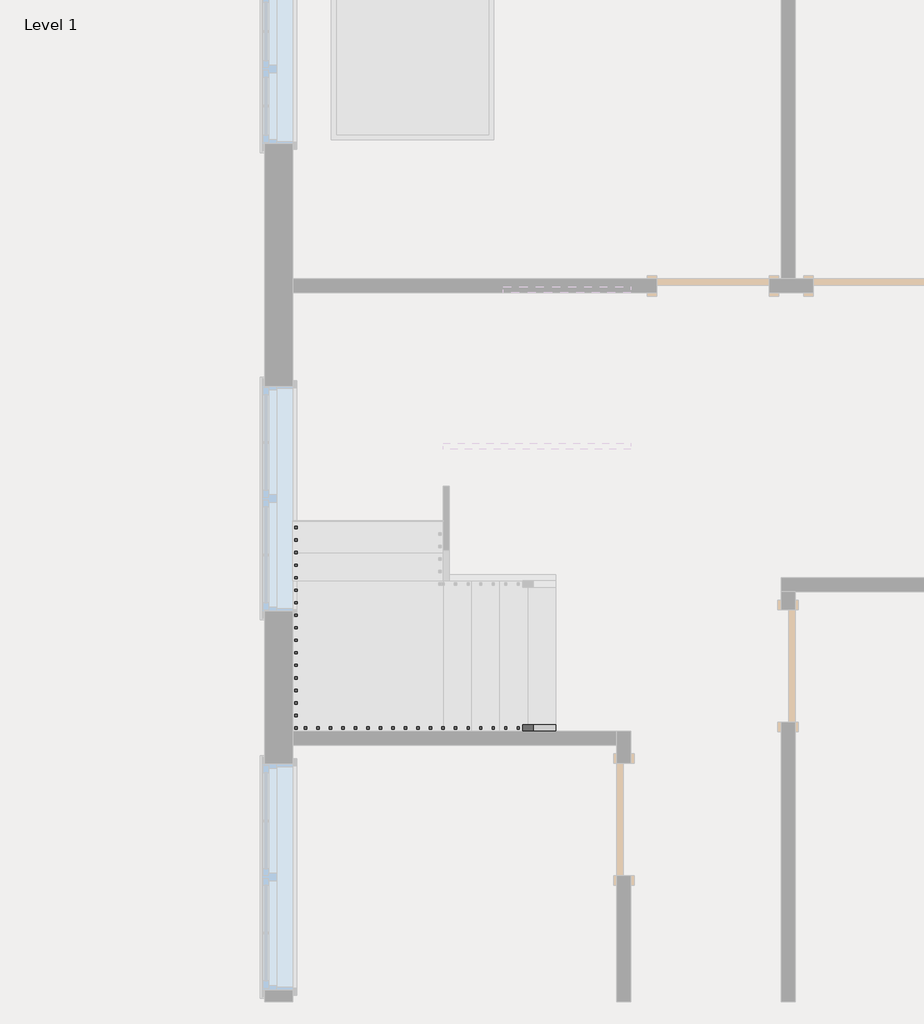
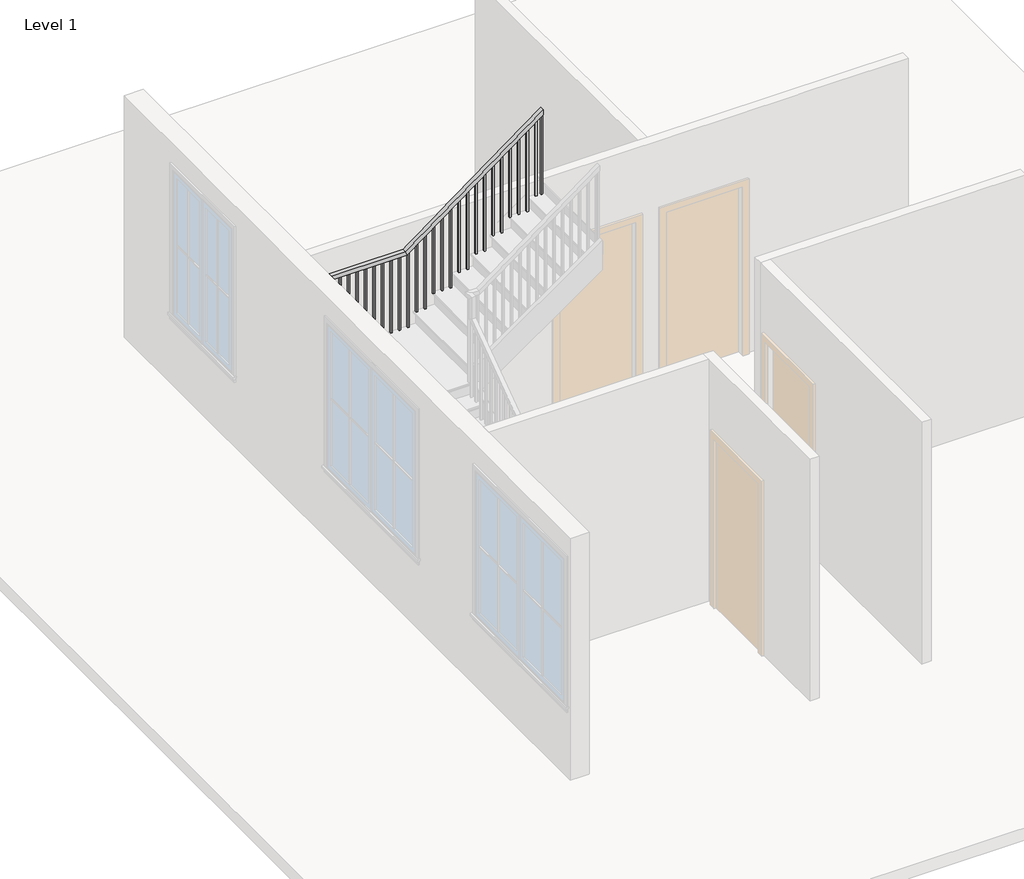
# One storey, part 2 of 3: 1 railing.
"""IFC4 building model written with IfcOpenShell, lengths in millimetres."""

from ifc_helpers import new_model, si_unit, frame, origin, place, context, project, spatial, polyline, outline, extrude, faceted_brep, element, save

model = new_model("IFC4")

# Units and contexts
model_context = context("Model", 3, world=origin())
ifc_project = project(units=[si_unit("LENGTHUNIT", "METRE", prefix="MILLI")], contexts=[model_context])

# Site, building, storey
site = spatial("IfcSite", under=ifc_project)
building = spatial("IfcBuilding", under=site)
storey = spatial("IfcBuildingStorey", under=building, Name="Level 1", Elevation=0.0)

# Railing
placement = place(None, origin())
element("IfcRailing", 1, ObjectType="Handrail - Rectangular", at=placement, inside=storey, context=model_context, shape_type="SolidModel", body=[
    faceted_brep([(-2683.1105391, -2741.0373761, 1074.8210526), (-2683.1105391, -2741.0373761, 1012.7605986), (-2683.1105391, -2690.2373761, 1012.7605986), (-2683.1105391, -2690.2373761, 1074.8210526), (-3698.24463, -2741.0373761, 1787.1958533), (-3714.290777, -2741.0373761, 1736.3958533), (-3714.290777, -2690.2373761, 1736.3958533), (-3698.24463, -2690.2373761, 1787.1958533), (-4816.7105391, -2741.0373761, 1787.1958533), (-4816.7105391, -2741.0373761, 1736.3958533), (-4765.9105391, -2690.2373761, 1736.3958533), (-4765.9105391, -2690.2373761, 1787.1958533), (-4816.7105391, -1646.8618205, 1787.1958533), (-4816.7105391, -1630.5188912, 1736.3958533), (-4765.9105391, -1630.5188912, 1736.3958533), (-4765.9105391, -1646.8618205, 1787.1958533), (-4816.7105391, -308.3947094, 2747.8181818), (-4816.7105391, -292.0517801, 2697.0181818), (-4765.9105391, -292.0517801, 2697.0181818), (-4765.9105391, -308.3947094, 2747.8181818), (-4816.7105391, 814.9626239, 2747.8181818), (-4816.7105391, 814.9626239, 2697.0181818), (-4765.9105391, 764.1626239, 2697.0181818), (-4765.9105391, 764.1626239, 2747.8181818), (-3721.871578, 814.9626239, 2747.8181818), (-3705.1770744, 814.9626239, 2697.0181818), (-3705.1770744, 764.1626239, 2697.0181818), (-3721.871578, 764.1626239, 2747.8181818), (-2073.5105391, 814.9626239, 3962.4), (-2073.5105391, 764.1626239, 3962.4), (-2073.5105391, 764.1626239, 3899.2987868), (-2073.5105391, 814.9626239, 3899.2987868)], [[[0, 1, 2, 3]], [[1, 0, 4, 5]], [[2, 1, 5, 6]], [[3, 2, 6, 7]], [[0, 3, 7, 4]], [[5, 4, 8, 9]], [[6, 5, 9, 10]], [[7, 6, 10, 11]], [[4, 7, 11, 8]], [[9, 8, 12, 13]], [[10, 9, 13, 14]], [[11, 10, 14, 15]], [[8, 11, 15, 12]], [[13, 12, 16, 17]], [[14, 13, 17, 18]], [[15, 14, 18, 19]], [[12, 15, 19, 16]], [[17, 16, 20, 21]], [[18, 17, 21, 22]], [[19, 18, 22, 23]], [[16, 19, 23, 20]], [[21, 20, 24, 25]], [[22, 21, 25, 26]], [[23, 22, 26, 27]], [[20, 23, 27, 24]], [[28, 29, 30, 31]], [[25, 24, 28, 31]], [[26, 25, 31, 30]], [[27, 26, 30, 29]], [[24, 27, 29, 28]]]),
    extrude(outline(polyline([(3836.1329974, -2159.2355391), (2887.5789474, -2159.2355391), (2887.5789474, -2140.1855391), (3850.1698395, -2140.1855391), (3836.1329974, -2159.2355391)])), frame((0.0, 780.0376239, 0.0), z_axis=(0.0, 1.0, 0.0), x_axis=(0.0, 0.0, 1.0)), (0.0, 0.0, 1.0), 19.05),
    extrude(outline(polyline([(3761.2698395, -2260.8355391), (2727.1578947, -2260.8355391), (2727.1578947, -2241.7855391), (3775.3066816, -2241.7855391), (3761.2698395, -2260.8355391)])), frame((0.0, 780.0376239, 0.0), z_axis=(0.0, 1.0, 0.0), x_axis=(0.0, 0.0, 1.0)), (0.0, 0.0, 1.0), 19.05),
    extrude(outline(polyline([(3686.4066816, -2362.4355391), (2727.1578947, -2362.4355391), (2727.1578947, -2343.3855391), (3700.4435237, -2343.3855391), (3686.4066816, -2362.4355391)])), frame((0.0, 780.0376239, 0.0), z_axis=(0.0, 1.0, 0.0), x_axis=(0.0, 0.0, 1.0)), (0.0, 0.0, 1.0), 19.05),
    extrude(outline(polyline([(3611.5435237, -2464.0355391), (2727.1578947, -2464.0355391), (2727.1578947, -2444.9855391), (3625.5803658, -2444.9855391), (3611.5435237, -2464.0355391)])), frame((0.0, 780.0376239, 0.0), z_axis=(0.0, 1.0, 0.0), x_axis=(0.0, 0.0, 1.0)), (0.0, 0.0, 1.0), 19.05),
    extrude(outline(polyline([(3536.6803658, -2565.6355391), (2566.7368421, -2565.6355391), (2566.7368421, -2546.5855391), (3550.7172079, -2546.5855391), (3536.6803658, -2565.6355391)])), frame((0.0, 780.0376239, 0.0), z_axis=(0.0, 1.0, 0.0), x_axis=(0.0, 0.0, 1.0)), (0.0, 0.0, 1.0), 19.05),
    extrude(outline(polyline([(3461.8172079, -2667.2355391), (2566.7368421, -2667.2355391), (2566.7368421, -2648.1855391), (3475.85405, -2648.1855391), (3461.8172079, -2667.2355391)])), frame((0.0, 780.0376239, 0.0), z_axis=(0.0, 1.0, 0.0), x_axis=(0.0, 0.0, 1.0)), (0.0, 0.0, 1.0), 19.05),
    extrude(outline(polyline([(3386.95405, -2768.8355391), (2406.3157895, -2768.8355391), (2406.3157895, -2749.7855391), (3400.9908921, -2749.7855391), (3386.95405, -2768.8355391)])), frame((0.0, 780.0376239, 0.0), z_axis=(0.0, 1.0, 0.0), x_axis=(0.0, 0.0, 1.0)), (0.0, 0.0, 1.0), 19.05),
    extrude(outline(polyline([(3312.0908921, -2870.4355391), (2406.3157895, -2870.4355391), (2406.3157895, -2851.3855391), (3326.1277342, -2851.3855391), (3312.0908921, -2870.4355391)])), frame((0.0, 780.0376239, 0.0), z_axis=(0.0, 1.0, 0.0), x_axis=(0.0, 0.0, 1.0)), (0.0, 0.0, 1.0), 19.05),
    extrude(outline(polyline([(3237.2277342, -2972.0355391), (2245.8947368, -2972.0355391), (2245.8947368, -2952.9855391), (3251.2645763, -2952.9855391), (3237.2277342, -2972.0355391)])), frame((0.0, 780.0376239, 0.0), z_axis=(0.0, 1.0, 0.0), x_axis=(0.0, 0.0, 1.0)), (0.0, 0.0, 1.0), 19.05),
    extrude(outline(polyline([(3162.3645763, -3073.6355391), (2245.8947368, -3073.6355391), (2245.8947368, -3054.5855391), (3176.4014184, -3054.5855391), (3162.3645763, -3073.6355391)])), frame((0.0, 780.0376239, 0.0), z_axis=(0.0, 1.0, 0.0), x_axis=(0.0, 0.0, 1.0)), (0.0, 0.0, 1.0), 19.05),
    extrude(outline(polyline([(3087.5014184, -3175.2355391), (2085.4736842, -3175.2355391), (2085.4736842, -3156.1855391), (3101.5382605, -3156.1855391), (3087.5014184, -3175.2355391)])), frame((0.0, 780.0376239, 0.0), z_axis=(0.0, 1.0, 0.0), x_axis=(0.0, 0.0, 1.0)), (0.0, 0.0, 1.0), 19.05),
    extrude(outline(polyline([(3012.6382605, -3276.8355391), (2085.4736842, -3276.8355391), (2085.4736842, -3257.7855391), (3026.6751026, -3257.7855391), (3012.6382605, -3276.8355391)])), frame((0.0, 780.0376239, 0.0), z_axis=(0.0, 1.0, 0.0), x_axis=(0.0, 0.0, 1.0)), (0.0, 0.0, 1.0), 19.05),
    extrude(outline(polyline([(2937.7751026, -3378.4355391), (2085.4736842, -3378.4355391), (2085.4736842, -3359.3855391), (2951.8119447, -3359.3855391), (2937.7751026, -3378.4355391)])), frame((0.0, 780.0376239, 0.0), z_axis=(0.0, 1.0, 0.0), x_axis=(0.0, 0.0, 1.0)), (0.0, 0.0, 1.0), 19.05),
    extrude(outline(polyline([(2862.9119447, -3480.0355391), (1925.0526316, -3480.0355391), (1925.0526316, -3460.9855391), (2876.9487868, -3460.9855391), (2862.9119447, -3480.0355391)])), frame((0.0, 780.0376239, 0.0), z_axis=(0.0, 1.0, 0.0), x_axis=(0.0, 0.0, 1.0)), (0.0, 0.0, 1.0), 19.05),
    extrude(outline(polyline([(2788.0487868, -3581.6355391), (1925.0526316, -3581.6355391), (1925.0526316, -3562.5855391), (2802.0856289, -3562.5855391), (2788.0487868, -3581.6355391)])), frame((0.0, 780.0376239, 0.0), z_axis=(0.0, 1.0, 0.0), x_axis=(0.0, 0.0, 1.0)), (0.0, 0.0, 1.0), 19.05),
    extrude(outline(polyline([(2713.1856289, -3683.2355391), (1764.6315789, -3683.2355391), (1764.6315789, -3664.1855391), (2727.222471, -3664.1855391), (2713.1856289, -3683.2355391)])), frame((0.0, 780.0376239, 0.0), z_axis=(0.0, 1.0, 0.0), x_axis=(0.0, 0.0, 1.0)), (0.0, 0.0, 1.0), 19.05),
    extrude(outline(polyline([(-3784.8355391, 799.0876239), (-3765.7855391, 799.0876239), (-3765.7855391, 780.0376239), (-3784.8355391, 780.0376239), (-3784.8355391, 799.0876239)])), frame((0.0, 0.0, 1764.6315789), z_axis=(0.0, 0.0, 1.0), x_axis=(1.0, 0.0, 0.0)), (0.0, 0.0, 1.0), 932.3866029),
    extrude(outline(polyline([(-3886.4355391, 799.0876239), (-3867.3855391, 799.0876239), (-3867.3855391, 780.0376239), (-3886.4355391, 780.0376239), (-3886.4355391, 799.0876239)])), frame((0.0, 0.0, 1764.6315789), z_axis=(0.0, 0.0, 1.0), x_axis=(1.0, 0.0, 0.0)), (0.0, 0.0, 1.0), 932.3866029),
    extrude(outline(polyline([(-3988.0355391, 799.0876239), (-3968.9855391, 799.0876239), (-3968.9855391, 780.0376239), (-3988.0355391, 780.0376239), (-3988.0355391, 799.0876239)])), frame((0.0, 0.0, 1764.6315789), z_axis=(0.0, 0.0, 1.0), x_axis=(1.0, 0.0, 0.0)), (0.0, 0.0, 1.0), 932.3866029),
    extrude(outline(polyline([(-4089.6355391, 799.0876239), (-4070.5855391, 799.0876239), (-4070.5855391, 780.0376239), (-4089.6355391, 780.0376239), (-4089.6355391, 799.0876239)])), frame((0.0, 0.0, 1764.6315789), z_axis=(0.0, 0.0, 1.0), x_axis=(1.0, 0.0, 0.0)), (0.0, 0.0, 1.0), 932.3866029),
    extrude(outline(polyline([(-4191.2355391, 799.0876239), (-4172.1855391, 799.0876239), (-4172.1855391, 780.0376239), (-4191.2355391, 780.0376239), (-4191.2355391, 799.0876239)])), frame((0.0, 0.0, 1764.6315789), z_axis=(0.0, 0.0, 1.0), x_axis=(1.0, 0.0, 0.0)), (0.0, 0.0, 1.0), 932.3866029),
    extrude(outline(polyline([(-4292.8355391, 799.0876239), (-4273.7855391, 799.0876239), (-4273.7855391, 780.0376239), (-4292.8355391, 780.0376239), (-4292.8355391, 799.0876239)])), frame((0.0, 0.0, 1764.6315789), z_axis=(0.0, 0.0, 1.0), x_axis=(1.0, 0.0, 0.0)), (0.0, 0.0, 1.0), 932.3866029),
    extrude(outline(polyline([(-4394.4355391, 799.0876239), (-4375.3855391, 799.0876239), (-4375.3855391, 780.0376239), (-4394.4355391, 780.0376239), (-4394.4355391, 799.0876239)])), frame((0.0, 0.0, 1764.6315789), z_axis=(0.0, 0.0, 1.0), x_axis=(1.0, 0.0, 0.0)), (0.0, 0.0, 1.0), 932.3866029),
    extrude(outline(polyline([(-4496.0355391, 799.0876239), (-4476.9855391, 799.0876239), (-4476.9855391, 780.0376239), (-4496.0355391, 780.0376239), (-4496.0355391, 799.0876239)])), frame((0.0, 0.0, 1764.6315789), z_axis=(0.0, 0.0, 1.0), x_axis=(1.0, 0.0, 0.0)), (0.0, 0.0, 1.0), 932.3866029),
    extrude(outline(polyline([(-4597.6355391, 799.0876239), (-4578.5855391, 799.0876239), (-4578.5855391, 780.0376239), (-4597.6355391, 780.0376239), (-4597.6355391, 799.0876239)])), frame((0.0, 0.0, 1764.6315789), z_axis=(0.0, 0.0, 1.0), x_axis=(1.0, 0.0, 0.0)), (0.0, 0.0, 1.0), 932.3866029),
    extrude(outline(polyline([(-4699.2355391, 799.0876239), (-4680.1855391, 799.0876239), (-4680.1855391, 780.0376239), (-4699.2355391, 780.0376239), (-4699.2355391, 799.0876239)])), frame((0.0, 0.0, 1764.6315789), z_axis=(0.0, 0.0, 1.0), x_axis=(1.0, 0.0, 0.0)), (0.0, 0.0, 1.0), 932.3866029),
    extrude(outline(polyline([(-4800.8355391, 729.2376239), (-4800.8355391, 748.2876239), (-4781.7855391, 748.2876239), (-4781.7855391, 729.2376239), (-4800.8355391, 729.2376239)])), frame((0.0, 0.0, 1764.6315789), z_axis=(0.0, 0.0, 1.0), x_axis=(1.0, 0.0, 0.0)), (0.0, 0.0, 1.0), 932.3866029),
    extrude(outline(polyline([(-4800.8355391, 627.6376239), (-4800.8355391, 646.6876239), (-4781.7855391, 646.6876239), (-4781.7855391, 627.6376239), (-4800.8355391, 627.6376239)])), frame((0.0, 0.0, 1764.6315789), z_axis=(0.0, 0.0, 1.0), x_axis=(1.0, 0.0, 0.0)), (0.0, 0.0, 1.0), 932.3866029),
    extrude(outline(polyline([(-4800.8355391, 526.0376239), (-4800.8355391, 545.0876239), (-4781.7855391, 545.0876239), (-4781.7855391, 526.0376239), (-4800.8355391, 526.0376239)])), frame((0.0, 0.0, 1764.6315789), z_axis=(0.0, 0.0, 1.0), x_axis=(1.0, 0.0, 0.0)), (0.0, 0.0, 1.0), 932.3866029),
    extrude(outline(polyline([(-4800.8355391, 424.4376239), (-4800.8355391, 443.4876239), (-4781.7855391, 443.4876239), (-4781.7855391, 424.4376239), (-4800.8355391, 424.4376239)])), frame((0.0, 0.0, 1764.6315789), z_axis=(0.0, 0.0, 1.0), x_axis=(1.0, 0.0, 0.0)), (0.0, 0.0, 1.0), 932.3866029),
    extrude(outline(polyline([(-4800.8355391, 322.8376239), (-4800.8355391, 341.8876239), (-4781.7855391, 341.8876239), (-4781.7855391, 322.8376239), (-4800.8355391, 322.8376239)])), frame((0.0, 0.0, 1764.6315789), z_axis=(0.0, 0.0, 1.0), x_axis=(1.0, 0.0, 0.0)), (0.0, 0.0, 1.0), 932.3866029),
    extrude(outline(polyline([(-4800.8355391, 221.2376239), (-4800.8355391, 240.2876239), (-4781.7855391, 240.2876239), (-4781.7855391, 221.2376239), (-4800.8355391, 221.2376239)])), frame((0.0, 0.0, 1764.6315789), z_axis=(0.0, 0.0, 1.0), x_axis=(1.0, 0.0, 0.0)), (0.0, 0.0, 1.0), 932.3866029),
    extrude(outline(polyline([(-4800.8355391, 119.6376239), (-4800.8355391, 138.6876239), (-4781.7855391, 138.6876239), (-4781.7855391, 119.6376239), (-4800.8355391, 119.6376239)])), frame((0.0, 0.0, 1764.6315789), z_axis=(0.0, 0.0, 1.0), x_axis=(1.0, 0.0, 0.0)), (0.0, 0.0, 1.0), 932.3866029),
    extrude(outline(polyline([(-4800.8355391, 18.0376239), (-4800.8355391, 37.0876239), (-4781.7855391, 37.0876239), (-4781.7855391, 18.0376239), (-4800.8355391, 18.0376239)])), frame((0.0, 0.0, 1764.6315789), z_axis=(0.0, 0.0, 1.0), x_axis=(1.0, 0.0, 0.0)), (0.0, 0.0, 1.0), 932.3866029),
    extrude(outline(polyline([(-4800.8355391, -83.5623761), (-4800.8355391, -64.5123761), (-4781.7855391, -64.5123761), (-4781.7855391, -83.5623761), (-4800.8355391, -83.5623761)])), frame((0.0, 0.0, 1764.6315789), z_axis=(0.0, 0.0, 1.0), x_axis=(1.0, 0.0, 0.0)), (0.0, 0.0, 1.0), 932.3866029),
    extrude(outline(polyline([(-4800.8355391, -185.1623761), (-4800.8355391, -166.1123761), (-4781.7855391, -166.1123761), (-4781.7855391, -185.1623761), (-4800.8355391, -185.1623761)])), frame((0.0, 0.0, 1764.6315789), z_axis=(0.0, 0.0, 1.0), x_axis=(1.0, 0.0, 0.0)), (0.0, 0.0, 1.0), 932.3866029),
    extrude(outline(polyline([(-4800.8355391, -286.7623761), (-4800.8355391, -267.7123761), (-4781.7855391, -267.7123761), (-4781.7855391, -286.7623761), (-4800.8355391, -286.7623761)])), frame((0.0, 0.0, 1764.6315789), z_axis=(0.0, 0.0, 1.0), x_axis=(1.0, 0.0, 0.0)), (0.0, 0.0, 1.0), 932.3866029),
    extrude(outline(polyline([(-369.3123761, 2641.5679933), (-369.3123761, 1764.6315789), (-388.3623761, 1764.6315789), (-388.3623761, 2627.8957445), (-369.3123761, 2641.5679933)])), frame((-4800.8355391, 0.0, 0.0), z_axis=(1.0, 0.0, 0.0), x_axis=(0.0, 1.0, 0.0)), (0.0, 0.0, 1.0), 19.05),
    extrude(outline(polyline([(-470.9123761, 2568.649333), (-470.9123761, 1604.2105263), (-489.9623761, 1604.2105263), (-489.9623761, 2554.9770842), (-470.9123761, 2568.649333)])), frame((-4800.8355391, 0.0, 0.0), z_axis=(1.0, 0.0, 0.0), x_axis=(0.0, 1.0, 0.0)), (0.0, 0.0, 1.0), 19.05),
    extrude(outline(polyline([(-572.5123761, 2495.7306727), (-572.5123761, 1604.2105263), (-591.5623761, 1604.2105263), (-591.5623761, 2482.0584239), (-572.5123761, 2495.7306727)])), frame((-4800.8355391, 0.0, 0.0), z_axis=(1.0, 0.0, 0.0), x_axis=(0.0, 1.0, 0.0)), (0.0, 0.0, 1.0), 19.05),
    extrude(outline(polyline([(-674.1123761, 2422.8120124), (-674.1123761, 1443.7894737), (-693.1623761, 1443.7894737), (-693.1623761, 2409.1397636), (-674.1123761, 2422.8120124)])), frame((-4800.8355391, 0.0, 0.0), z_axis=(1.0, 0.0, 0.0), x_axis=(0.0, 1.0, 0.0)), (0.0, 0.0, 1.0), 19.05),
    extrude(outline(polyline([(-775.7123761, 2349.8933521), (-775.7123761, 1443.7894737), (-794.7623761, 1443.7894737), (-794.7623761, 2336.2211033), (-775.7123761, 2349.8933521)])), frame((-4800.8355391, 0.0, 0.0), z_axis=(1.0, 0.0, 0.0), x_axis=(0.0, 1.0, 0.0)), (0.0, 0.0, 1.0), 19.05),
    extrude(outline(polyline([(-877.3123761, 2276.9746919), (-877.3123761, 1283.3684211), (-896.3623761, 1283.3684211), (-896.3623761, 2263.302443), (-877.3123761, 2276.9746919)])), frame((-4800.8355391, 0.0, 0.0), z_axis=(1.0, 0.0, 0.0), x_axis=(0.0, 1.0, 0.0)), (0.0, 0.0, 1.0), 19.05),
    extrude(outline(polyline([(-978.9123761, 2204.0560316), (-978.9123761, 1283.3684211), (-997.9623761, 1283.3684211), (-997.9623761, 2190.3837828), (-978.9123761, 2204.0560316)])), frame((-4800.8355391, 0.0, 0.0), z_axis=(1.0, 0.0, 0.0), x_axis=(0.0, 1.0, 0.0)), (0.0, 0.0, 1.0), 19.05),
    extrude(outline(polyline([(-1080.5123761, 2131.1373713), (-1080.5123761, 1122.9473684), (-1099.5623761, 1122.9473684), (-1099.5623761, 2117.4651225), (-1080.5123761, 2131.1373713)])), frame((-4800.8355391, 0.0, 0.0), z_axis=(1.0, 0.0, 0.0), x_axis=(0.0, 1.0, 0.0)), (0.0, 0.0, 1.0), 19.05),
    extrude(outline(polyline([(-1182.1123761, 2058.218711), (-1182.1123761, 1122.9473684), (-1201.1623761, 1122.9473684), (-1201.1623761, 2044.5464622), (-1182.1123761, 2058.218711)])), frame((-4800.8355391, 0.0, 0.0), z_axis=(1.0, 0.0, 0.0), x_axis=(0.0, 1.0, 0.0)), (0.0, 0.0, 1.0), 19.05),
    extrude(outline(polyline([(-1283.7123761, 1985.3000507), (-1283.7123761, 1122.9473684), (-1302.7623761, 1122.9473684), (-1302.7623761, 1971.6278019), (-1283.7123761, 1985.3000507)])), frame((-4800.8355391, 0.0, 0.0), z_axis=(1.0, 0.0, 0.0), x_axis=(0.0, 1.0, 0.0)), (0.0, 0.0, 1.0), 19.05),
    extrude(outline(polyline([(-1385.3123761, 1912.3813904), (-1385.3123761, 962.5263158), (-1404.3623761, 962.5263158), (-1404.3623761, 1898.7091416), (-1385.3123761, 1912.3813904)])), frame((-4800.8355391, 0.0, 0.0), z_axis=(1.0, 0.0, 0.0), x_axis=(0.0, 1.0, 0.0)), (0.0, 0.0, 1.0), 19.05),
    extrude(outline(polyline([(-1486.9123761, 1839.4627301), (-1486.9123761, 962.5263158), (-1505.9623761, 962.5263158), (-1505.9623761, 1825.7904813), (-1486.9123761, 1839.4627301)])), frame((-4800.8355391, 0.0, 0.0), z_axis=(1.0, 0.0, 0.0), x_axis=(0.0, 1.0, 0.0)), (0.0, 0.0, 1.0), 19.05),
    extrude(outline(polyline([(-1588.5123761, 1766.5440698), (-1588.5123761, 802.1052632), (-1607.5623761, 802.1052632), (-1607.5623761, 1752.871821), (-1588.5123761, 1766.5440698)])), frame((-4800.8355391, 0.0, 0.0), z_axis=(1.0, 0.0, 0.0), x_axis=(0.0, 1.0, 0.0)), (0.0, 0.0, 1.0), 19.05),
    extrude(outline(polyline([(-4800.8355391, -1709.1623761), (-4800.8355391, -1690.1123761), (-4781.7855391, -1690.1123761), (-4781.7855391, -1709.1623761), (-4800.8355391, -1709.1623761)])), frame((0.0, 0.0, 802.1052632), z_axis=(0.0, 0.0, 1.0), x_axis=(1.0, 0.0, 0.0)), (0.0, 0.0, 1.0), 934.2905901),
    extrude(outline(polyline([(-4800.8355391, -1810.7623761), (-4800.8355391, -1791.7123761), (-4781.7855391, -1791.7123761), (-4781.7855391, -1810.7623761), (-4800.8355391, -1810.7623761)])), frame((0.0, 0.0, 802.1052632), z_axis=(0.0, 0.0, 1.0), x_axis=(1.0, 0.0, 0.0)), (0.0, 0.0, 1.0), 934.2905901),
    extrude(outline(polyline([(-4800.8355391, -1912.3623761), (-4800.8355391, -1893.3123761), (-4781.7855391, -1893.3123761), (-4781.7855391, -1912.3623761), (-4800.8355391, -1912.3623761)])), frame((0.0, 0.0, 802.1052632), z_axis=(0.0, 0.0, 1.0), x_axis=(1.0, 0.0, 0.0)), (0.0, 0.0, 1.0), 934.2905901),
    extrude(outline(polyline([(-4800.8355391, -2013.9623761), (-4800.8355391, -1994.9123761), (-4781.7855391, -1994.9123761), (-4781.7855391, -2013.9623761), (-4800.8355391, -2013.9623761)])), frame((0.0, 0.0, 802.1052632), z_axis=(0.0, 0.0, 1.0), x_axis=(1.0, 0.0, 0.0)), (0.0, 0.0, 1.0), 934.2905901),
    extrude(outline(polyline([(-4800.8355391, -2115.5623761), (-4800.8355391, -2096.5123761), (-4781.7855391, -2096.5123761), (-4781.7855391, -2115.5623761), (-4800.8355391, -2115.5623761)])), frame((0.0, 0.0, 802.1052632), z_axis=(0.0, 0.0, 1.0), x_axis=(1.0, 0.0, 0.0)), (0.0, 0.0, 1.0), 934.2905901),
    extrude(outline(polyline([(-4800.8355391, -2217.1623761), (-4800.8355391, -2198.1123761), (-4781.7855391, -2198.1123761), (-4781.7855391, -2217.1623761), (-4800.8355391, -2217.1623761)])), frame((0.0, 0.0, 802.1052632), z_axis=(0.0, 0.0, 1.0), x_axis=(1.0, 0.0, 0.0)), (0.0, 0.0, 1.0), 934.2905901),
    extrude(outline(polyline([(-4800.8355391, -2318.7623761), (-4800.8355391, -2299.7123761), (-4781.7855391, -2299.7123761), (-4781.7855391, -2318.7623761), (-4800.8355391, -2318.7623761)])), frame((0.0, 0.0, 802.1052632), z_axis=(0.0, 0.0, 1.0), x_axis=(1.0, 0.0, 0.0)), (0.0, 0.0, 1.0), 934.2905901),
    extrude(outline(polyline([(-4800.8355391, -2420.3623761), (-4800.8355391, -2401.3123761), (-4781.7855391, -2401.3123761), (-4781.7855391, -2420.3623761), (-4800.8355391, -2420.3623761)])), frame((0.0, 0.0, 802.1052632), z_axis=(0.0, 0.0, 1.0), x_axis=(1.0, 0.0, 0.0)), (0.0, 0.0, 1.0), 934.2905901),
    extrude(outline(polyline([(-4800.8355391, -2521.9623761), (-4800.8355391, -2502.9123761), (-4781.7855391, -2502.9123761), (-4781.7855391, -2521.9623761), (-4800.8355391, -2521.9623761)])), frame((0.0, 0.0, 802.1052632), z_axis=(0.0, 0.0, 1.0), x_axis=(1.0, 0.0, 0.0)), (0.0, 0.0, 1.0), 934.2905901),
    extrude(outline(polyline([(-4800.8355391, -2623.5623761), (-4800.8355391, -2604.5123761), (-4781.7855391, -2604.5123761), (-4781.7855391, -2623.5623761), (-4800.8355391, -2623.5623761)])), frame((0.0, 0.0, 802.1052632), z_axis=(0.0, 0.0, 1.0), x_axis=(1.0, 0.0, 0.0)), (0.0, 0.0, 1.0), 934.2905901),
    extrude(outline(polyline([(-4705.5855391, -2725.1623761), (-4724.6355391, -2725.1623761), (-4724.6355391, -2706.1123761), (-4705.5855391, -2706.1123761), (-4705.5855391, -2725.1623761)])), frame((0.0, 0.0, 802.1052632), z_axis=(0.0, 0.0, 1.0), x_axis=(1.0, 0.0, 0.0)), (0.0, 0.0, 1.0), 934.2905901),
    extrude(outline(polyline([(-4603.9855391, -2725.1623761), (-4623.0355391, -2725.1623761), (-4623.0355391, -2706.1123761), (-4603.9855391, -2706.1123761), (-4603.9855391, -2725.1623761)])), frame((0.0, 0.0, 802.1052632), z_axis=(0.0, 0.0, 1.0), x_axis=(1.0, 0.0, 0.0)), (0.0, 0.0, 1.0), 934.2905901),
    extrude(outline(polyline([(-4502.3855391, -2725.1623761), (-4521.4355391, -2725.1623761), (-4521.4355391, -2706.1123761), (-4502.3855391, -2706.1123761), (-4502.3855391, -2725.1623761)])), frame((0.0, 0.0, 802.1052632), z_axis=(0.0, 0.0, 1.0), x_axis=(1.0, 0.0, 0.0)), (0.0, 0.0, 1.0), 934.2905901),
    extrude(outline(polyline([(-4400.7855391, -2725.1623761), (-4419.8355391, -2725.1623761), (-4419.8355391, -2706.1123761), (-4400.7855391, -2706.1123761), (-4400.7855391, -2725.1623761)])), frame((0.0, 0.0, 802.1052632), z_axis=(0.0, 0.0, 1.0), x_axis=(1.0, 0.0, 0.0)), (0.0, 0.0, 1.0), 934.2905901),
    extrude(outline(polyline([(-4299.1855391, -2725.1623761), (-4318.2355391, -2725.1623761), (-4318.2355391, -2706.1123761), (-4299.1855391, -2706.1123761), (-4299.1855391, -2725.1623761)])), frame((0.0, 0.0, 802.1052632), z_axis=(0.0, 0.0, 1.0), x_axis=(1.0, 0.0, 0.0)), (0.0, 0.0, 1.0), 934.2905901),
    extrude(outline(polyline([(-4197.5855391, -2725.1623761), (-4216.6355391, -2725.1623761), (-4216.6355391, -2706.1123761), (-4197.5855391, -2706.1123761), (-4197.5855391, -2725.1623761)])), frame((0.0, 0.0, 802.1052632), z_axis=(0.0, 0.0, 1.0), x_axis=(1.0, 0.0, 0.0)), (0.0, 0.0, 1.0), 934.2905901),
    extrude(outline(polyline([(-4095.9855391, -2725.1623761), (-4115.0355391, -2725.1623761), (-4115.0355391, -2706.1123761), (-4095.9855391, -2706.1123761), (-4095.9855391, -2725.1623761)])), frame((0.0, 0.0, 802.1052632), z_axis=(0.0, 0.0, 1.0), x_axis=(1.0, 0.0, 0.0)), (0.0, 0.0, 1.0), 934.2905901),
    extrude(outline(polyline([(-3994.3855391, -2725.1623761), (-4013.4355391, -2725.1623761), (-4013.4355391, -2706.1123761), (-3994.3855391, -2706.1123761), (-3994.3855391, -2725.1623761)])), frame((0.0, 0.0, 802.1052632), z_axis=(0.0, 0.0, 1.0), x_axis=(1.0, 0.0, 0.0)), (0.0, 0.0, 1.0), 934.2905901),
    extrude(outline(polyline([(-3892.7855391, -2725.1623761), (-3911.8355391, -2725.1623761), (-3911.8355391, -2706.1123761), (-3892.7855391, -2706.1123761), (-3892.7855391, -2725.1623761)])), frame((0.0, 0.0, 802.1052632), z_axis=(0.0, 0.0, 1.0), x_axis=(1.0, 0.0, 0.0)), (0.0, 0.0, 1.0), 934.2905901),
    extrude(outline(polyline([(-3791.1855391, -2725.1623761), (-3810.2355391, -2725.1623761), (-3810.2355391, -2706.1123761), (-3791.1855391, -2706.1123761), (-3791.1855391, -2725.1623761)])), frame((0.0, 0.0, 802.1052632), z_axis=(0.0, 0.0, 1.0), x_axis=(1.0, 0.0, 0.0)), (0.0, 0.0, 1.0), 934.2905901),
    extrude(outline(polyline([(-3689.5855391, -2725.1623761), (-3708.6355391, -2725.1623761), (-3708.6355391, -2706.1123761), (-3689.5855391, -2706.1123761), (-3689.5855391, -2725.1623761)])), frame((0.0, 0.0, 802.1052632), z_axis=(0.0, 0.0, 1.0), x_axis=(1.0, 0.0, 0.0)), (0.0, 0.0, 1.0), 934.2905901),
    extrude(outline(polyline([(1661.1290196, -3607.0355391), (802.1052632, -3607.0355391), (802.1052632, -3587.9855391), (1647.7605986, -3587.9855391), (1661.1290196, -3607.0355391)])), frame((0.0, -2725.1623761, 0.0), z_axis=(0.0, 1.0, 0.0), x_axis=(0.0, 0.0, 1.0)), (0.0, 0.0, 1.0), 19.05),
    extrude(outline(polyline([(1589.830774, -3505.4355391), (641.6842105, -3505.4355391), (641.6842105, -3486.3855391), (1576.462353, -3486.3855391), (1589.830774, -3505.4355391)])), frame((0.0, -2725.1623761, 0.0), z_axis=(0.0, 1.0, 0.0), x_axis=(0.0, 0.0, 1.0)), (0.0, 0.0, 1.0), 19.05),
    extrude(outline(polyline([(1518.5325284, -3403.8355391), (641.6842105, -3403.8355391), (641.6842105, -3384.7855391), (1505.1641074, -3384.7855391), (1518.5325284, -3403.8355391)])), frame((0.0, -2725.1623761, 0.0), z_axis=(0.0, 1.0, 0.0), x_axis=(0.0, 0.0, 1.0)), (0.0, 0.0, 1.0), 19.05),
    extrude(outline(polyline([(1447.2342828, -3302.2355391), (481.2631579, -3302.2355391), (481.2631579, -3283.1855391), (1433.8658617, -3283.1855391), (1447.2342828, -3302.2355391)])), frame((0.0, -2725.1623761, 0.0), z_axis=(0.0, 1.0, 0.0), x_axis=(0.0, 0.0, 1.0)), (0.0, 0.0, 1.0), 19.05),
    extrude(outline(polyline([(1375.9360372, -3200.6355391), (481.2631579, -3200.6355391), (481.2631579, -3181.5855391), (1362.5676161, -3181.5855391), (1375.9360372, -3200.6355391)])), frame((0.0, -2725.1623761, 0.0), z_axis=(0.0, 1.0, 0.0), x_axis=(0.0, 0.0, 1.0)), (0.0, 0.0, 1.0), 19.05),
    extrude(outline(polyline([(1304.6377916, -3099.0355391), (320.8421053, -3099.0355391), (320.8421053, -3079.9855391), (1291.2693705, -3079.9855391), (1304.6377916, -3099.0355391)])), frame((0.0, -2725.1623761, 0.0), z_axis=(0.0, 1.0, 0.0), x_axis=(0.0, 0.0, 1.0)), (0.0, 0.0, 1.0), 19.05),
    extrude(outline(polyline([(1233.3395459, -2997.4355391), (320.8421053, -2997.4355391), (320.8421053, -2978.3855391), (1219.9711249, -2978.3855391), (1233.3395459, -2997.4355391)])), frame((0.0, -2725.1623761, 0.0), z_axis=(0.0, 1.0, 0.0), x_axis=(0.0, 0.0, 1.0)), (0.0, 0.0, 1.0), 19.05),
    extrude(outline(polyline([(1162.0413003, -2895.8355391), (160.4210526, -2895.8355391), (160.4210526, -2876.7855391), (1148.6728793, -2876.7855391), (1162.0413003, -2895.8355391)])), frame((0.0, -2725.1623761, 0.0), z_axis=(0.0, 1.0, 0.0), x_axis=(0.0, 0.0, 1.0)), (0.0, 0.0, 1.0), 19.05),
    extrude(outline(polyline([(1090.7430547, -2794.2355391), (160.4210526, -2794.2355391), (160.4210526, -2775.1855391), (1077.3746337, -2775.1855391), (1090.7430547, -2794.2355391)])), frame((0.0, -2725.1623761, 0.0), z_axis=(0.0, 1.0, 0.0), x_axis=(0.0, 0.0, 1.0)), (0.0, 0.0, 1.0), 19.05),
    extrude(outline(polyline([(-4800.8355391, 780.0376239), (-4800.8355391, 799.0876239), (-4781.7855391, 799.0876239), (-4781.7855391, 780.0376239), (-4800.8355391, 780.0376239)])), frame((0.0, 0.0, 1764.6315789), z_axis=(0.0, 0.0, 1.0), x_axis=(1.0, 0.0, 0.0)), (0.0, 0.0, 1.0), 932.3866029),
    extrude(outline(polyline([(-4781.7855391, -2725.1623761), (-4800.8355391, -2725.1623761), (-4800.8355391, -2706.1123761), (-4781.7855391, -2706.1123761), (-4781.7855391, -2725.1623761)])), frame((0.0, 0.0, 802.1052632), z_axis=(0.0, 0.0, 1.0), x_axis=(1.0, 0.0, 0.0)), (0.0, 0.0, 1.0), 934.2905901),
    extrude(outline(polyline([(3885.2619447, -2092.5605391), (2887.5789474, -2092.5605391), (2887.5789474, -2073.5105391), (3899.2987868, -2073.5105391), (3885.2619447, -2092.5605391)])), frame((0.0, 780.0376239, 0.0), z_axis=(0.0, 1.0, 0.0), x_axis=(0.0, 0.0, 1.0)), (0.0, 0.0, 1.0), 19.05),
    extrude(outline(polyline([(1026.1290196, -2702.1605391), (160.4210526, -2702.1605391), (160.4210526, -2683.1105391), (1012.7605986, -2683.1105391), (1026.1290196, -2702.1605391)])), frame((0.0, -2725.1623761, 0.0), z_axis=(0.0, 1.0, 0.0), x_axis=(0.0, 0.0, 1.0)), (0.0, 0.0, 1.0), 19.05),
])

save(model, "model.ifc")

# Revit data of these elements
# Type "Handrail - Rectangular"
#   Assembly Code = "C2010400"
#   built-in parameter 1008612 = 0.0416667 (stored number, unit not read)
#   built-in parameter 1008611 = 0.0416667 (stored number, unit not read)
#   built-in parameter 1008609 = 0.333333 (stored number, unit not read)
#   built-in parameter 1008604 = 0.166667 (stored number, unit not read)
#   built-in parameter 1008603 = 0.166667 (stored number, unit not read)
#   Railing Height = 3' - 0"
#   built-in parameter 1008630 = 2
#   built-in parameter 1008610 = 2
#   built-in parameter 1008618 = Baluster - Square : 3/4"
# Element 1 (IfcRailing, "Handrail - Rectangular")
#   Phase Created = New Construction
